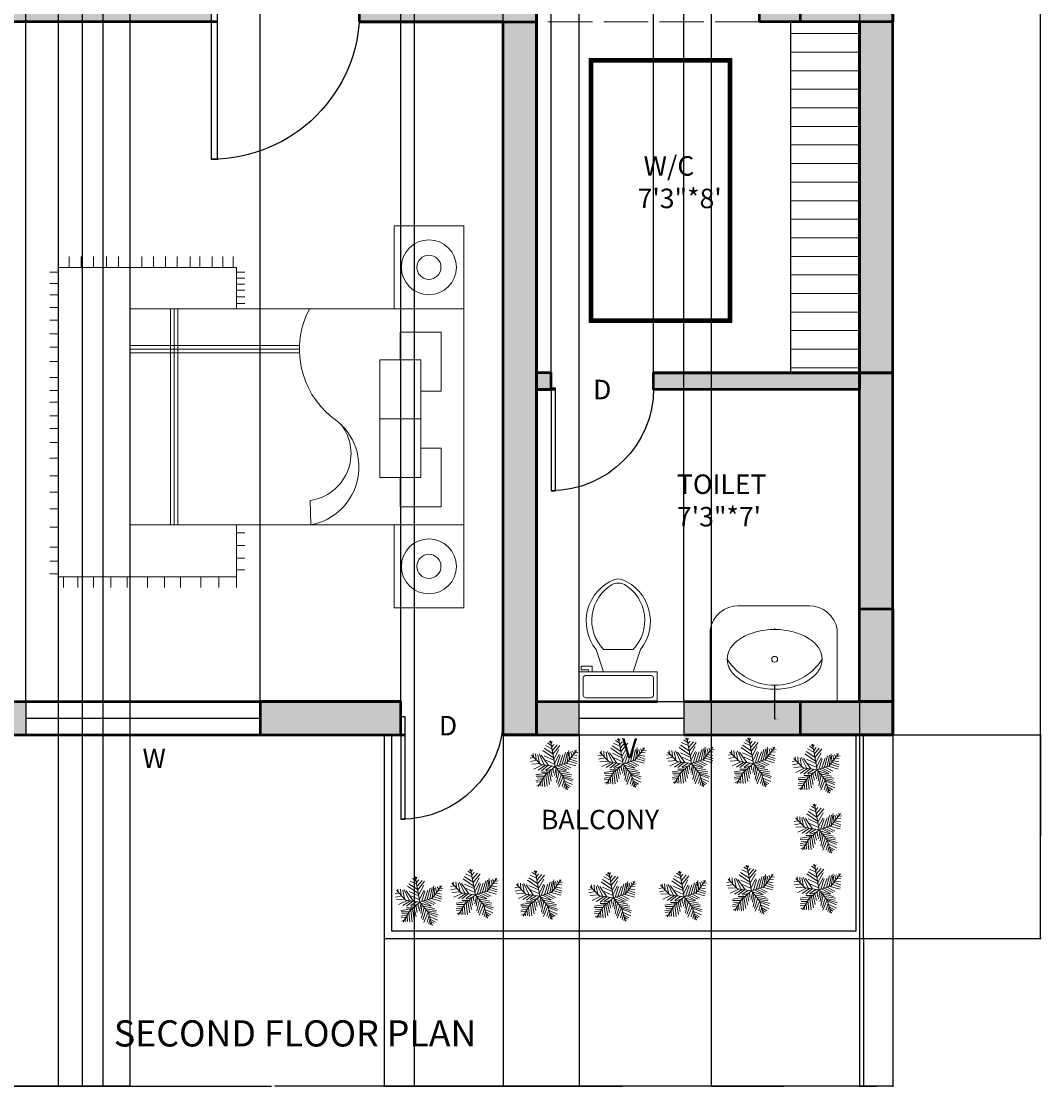
# Model space of a CAD drawing. Units: inches. Extents: x 2494 to 2908, y 1051 to 1885.
# Tile 2 of 7: x 2634 to 2908, y 1051 to 1338. Entities that reach past the tile are written whole.
import ezdxf

# ---------------------------------------------------------------- set-up
doc = ezdxf.new("R2010")
doc.units = ezdxf.units.IN
doc.linetypes.add('ACAD_ISO02W100', pattern=[15, 12, -3])
for name, color, linetype, lineweight in [('A-ANNO-DIMS', 2, 'Continuous', 18), ('A-ANNO-IDEN', 130, 'Continuous', 18), ('A-ANNO-TEXT', 130, 'Continuous', 35), ('A-AREA-IDEN', 130, 'Continuous', 18), ('A-COLS-PATT', 200, 'Continuous', 13), ('A-FLOR-CASE', 230, 'Continuous', 25), ('A-FLOR-FIXT', 230, 'Continuous', 18), ('A-FLOR-HRAL', 140, 'Continuous', 25), ('A-FURN-PATT', 230, 'Continuous', 13), ('A-WALL-OVHD', 140, 'ACAD_ISO02W100', 18), ('A-WALL-PATT', 140, 'Continuous', 13), ('COLUMN', 200, 'Continuous', 50), ('DOOR', 50, 'Continuous', 25), ('FUR', 230, 'Continuous', 18), ('TREE', 100, 'Continuous', 13), ('WALL', 140, 'Continuous', 50), ('WIND', 210, 'Continuous', 25)]:
    doc.layers.add(name, color=color, linetype=linetype, lineweight=lineweight)
doc.styles.get("Standard").update_dxf_attribs({"font": 'arial.ttf'})
doc.dimstyles.get("Standard").update_dxf_attribs({"dimtxt": 0.18, "dimasz": 0.18, "dimexe": 0.18, "dimexo": 0.0625, "dimgap": 0.09, "dimtad": 0, "dimtih": 1, "dimtoh": 1, "dimdec": 4, "dimzin": 0, "dimdsep": 46, "dimtxsty": 'Standard', "dimcen": 0.09, "dimadec": 0, "dimazin": 0, "dimtfac": 1, "dimtdec": 4, "dimtofl": 0, "dimtmove": 0, "dimatfit": 3, "dimfxl": 1, "dimtolj": 1, "dimtzin": 0, "dimarcsym": 0})

# ---------------------------------------------------------------- blocks, each defined once
blk = doc.blocks.new('*U6')
for p, q in [((-8.737, 47.138), (-17.069, 52.711)), ((-10.186, 53.64), (-13.084, 55.962)), ((0, 0), (-10.5, 57)), ((-9.099, 51.782), (-6.563, 55.962)), ((-7.65, 43.423), (-2.578, 49.46)), ((-5.839, 35.992), (4.667, 48.067)), ((-31.5, 4.5), (-52.5, 25.5)), ((-48.585, 21.131), (-49.309, 29.026)), ((-43.513, 28.561), (-42.427, 15.558)), ((-38.442, 26.239), (-34.819, 7.663)), ((-35.544, 28.097), (-24.314, 3.947)), ((-14.533, 2.09), (-30.834, 25.31)), ((-3.665, 19.273), (-27.574, 35.527)), ((-5.114, 28.097), (-24.676, 40.636)), ((-24.314, 23.917), (-2.941, 13.7)), ((-7.288, 39.707), (-21.778, 46.673)), ((-5.114, 27.632), (10.463, 46.673)), ((-2.941, 16.486), (8.652, 37.85)), ((-1.129, 6.734), (9.014, 26.704)), ((3.942, 1.625), (11.187, 24.381)), ((10.101, 3.483), (17.708, 26.239)), ((16.259, 5.805), (23.142, 31.348)), ((22.055, 7.198), (27.489, 32.277)), ((27, 9), (48, 36)), ((27.127, 9.056), (31.112, 35.992)), ((31.836, 30.883), (32.561, 16.486)), ((35.096, 32.741), (37.27, 22.524)), ((38.719, 34.134), (41.979, 28.561)), ((40.53, 25.775), (48.862, 24.846)), ((43.791, 29.954), (51.036, 30.883)), ((44.153, 36.456), (45.239, 32.741)), ((-47.498, 19.737), (-55.83, 18.344)), ((-40.615, 13.7), (-55.105, 10.913)), ((-33.37, 6.269), (-52.207, 5.34)), ((-28.299, 3.483), (-47.86, -5.805)), ((-21.416, 3.018), (-38.079, -8.128)), ((0, 0), (-31.5, 4.5)), ((-15.982, 2.09), (-30.11, -9.521)), ((0, 0), (-22.5, -19.5)), ((-6.563, 1.161), (-21.416, -8.128)), ((-20.691, 13.7), (-1.129, 4.876)), ((0, 0), (27, 9)), ((0, 0), (18, -22.5)), ((6.478, 1.625), (26.04, -8.592)), ((11.187, 3.483), (30.749, -5.805)), ((18.07, 5.805), (35.096, -3.483)), ((24.229, 7.663), (46.688, 1.625)), ((29.662, 12.307), (48.137, 6.269)), ((33.285, 16.486), (48.862, 10.913)), ((36.183, 19.737), (48.137, 17.88)), ((-17.431, -15.094), (-42.789, -18.809)), ((-24.314, -21.596), (-42.427, -22.06)), ((-22.5, -19.5), (-37.5, -45)), ((-15.257, -12.772), (-30.11, -12.772)), ((-20.691, -18.345), (-17.793, -44.352)), ((-6.563, -5.805), (-19.967, -9.985)), ((-17.069, -15.094), (-12.721, -40.172)), ((-13.446, -11.378), (-8.737, -32.741)), ((-9.461, -8.592), (-6.201, -23.453)), ((-4.752, -3.483), (-3.665, -14.629)), ((2.493, -3.019), (-1.491, -20.202)), ((1.769, -2.555), (24.229, -9.521)), ((5.029, -6.27), (2.131, -25.775)), ((9.014, -11.378), (3.58, -35.992)), ((14.085, -16.951), (6.478, -40.172)), ((7.565, -9.056), (32.198, -14.629)), ((18.07, -22.524), (8.289, -45.745)), ((12.274, -15.094), (36.907, -18.809)), ((16.259, -19.738), (36.183, -22.989)), ((18, -22.5), (27, -52.5)), ((18.433, -22.524), (40.53, -29.026)), ((-28.299, -29.026), (-42.789, -31.348)), ((-30.834, -34.135), (-42.427, -35.528)), ((-34.457, -39.708), (-40.978, -42.494)), ((-26.849, -26.24), (-40.253, -25.775)), ((-32.646, -36.921), (-31.921, -44.352)), ((-29.023, -30.884), (-27.936, -43.887)), ((-25.038, -23.918), (-22.865, -45.281)), ((20.244, -30.419), (15.897, -44.816)), ((19.157, -25.311), (38.719, -33.206)), ((22.78, -37.85), (19.519, -48.532)), ((21.331, -32.741), (39.081, -40.636)), ((22.78, -38.314), (34.372, -44.816)), ((24.591, -45.745), (23.142, -50.854)), ((24.591, -43.423), (30.749, -47.603)), ((26.764, -49.925), (28.213, -50.854))]:
    blk.add_line(p, q)
blk = doc.blocks.new('*U2')
for p, q in [((0, 0), (0, -6)), ((40, 0), (40, -6))]:
    blk.add_line(p, q)
blk.add_lwpolyline([(0, 0), (0, 40), (1.75, 40), (1.75, 0)], close=True)
blk.add_arc((0, 0), 40, 0, 90)
blk = doc.blocks.new('*U4')
for p, q in [((9.5, -6), (9.5, -2)), ((-10, -8.5), (-8, -8.5)), ((-10, -9.5), (-10, -8.5)), ((-8, -8.5), (-8, -8)), ((-7, -8), (-7, -9.5)), ((-4, -8), (-6, -14)), ((4, -8), (6, -14)), ((-7, -9.5), (-10, -9.5)), ((4, -14), (-4, -14))]:
    blk.add_line(p, q)
blk.add_lwpolyline([(10.5, -8), (10.5, 0), (-10.5, 0), (-10.5, -8)], close=True)
for points in [[(-9.5, -2), (-9.5, -6)], [(8.5, -1), (-8.5, -1)], [(-8.5, -7), (8.5, -7)]]:
    blk.add_lwpolyline(points)
for centre, radius, start, end in [((-8.62, -1.88), 0.884, 81.8699, 188.1301), ((8.62, -1.88), 0.884, 351.8699, 98.1301), ((-8.62, -6.12), 0.884, 171.8699, 278.1301), ((8.62, -6.12), 0.884, 261.8699, 8.1301), ((3.52, -21.58), 12.17, 141.4691, 247.9714), ((4.2, -21.82), 11.33, 136.3677, 238.9468), ((-3.52, -21.58), 12.17, 292.0284, 38.5307), ((-4.2, -21.82), 11.33, 301.053, 43.6321), ((0, -27.88), 4, 245.7318, 294.2682), ((0, -29), 4, 254.8605, 285.1395)]:
    blk.add_arc(centre, radius, start, end)
blk = doc.blocks.new('BED-DOUBLE')
for p, q in [((10.93, 58.24), (10.93, 0)), ((11.93, 58.24), (11.93, 0)), ((12.93, 58.24), (12.93, 0)), ((45.66, 48.34), (0, 48.34)), ((45.66, 47.34), (0, 47.34)), ((45.66, 46.34), (0, 46.34)), ((67.33, 28.6), (78.31, 28.6)), ((48.68, 0), (48.5, 6.63))]:
    blk.add_line(p, q)
for points in [[(89.88, 0), (0, 0), (0, 58.24), (89.88, 58.24)], [(78.31, 44.44), (67.33, 44.44), (67.33, 12.76), (78.31, 12.76)], [(67.33, 28.6), (78.31, 28.6), (78.31, 44.44), (67.33, 44.44)], [(67.33, 12.76), (78.31, 12.76), (78.31, 28.6), (67.33, 28.6)]]:
    blk.add_lwpolyline(points, close=True)
for points in [[(78.31, 36.06), (83.8, 36.06), (83.8, 51.9), (72.82, 51.9), (72.82, 44.44)], [(72.82, 12.76), (72.82, 4.84), (83.8, 4.84), (83.8, 20.68), (78.31, 20.68)]]:
    blk.add_lwpolyline(points)
for centre, radius, start, end in [((69.31, 47.34), 23.65, 152.5545, 230.8062), ((45.78, 15.63), 15.89, 280.497, 57.3115), ((46.81, 19.24), 12.73, 277.6511, 37.2925)]:
    blk.add_arc(centre, radius, start, end)
blk = doc.blocks.new('NIGHTSTAND-WITH-LAMP')
blk.add_lwpolyline([(18.73, 0), (0, 0), (0, 22.3), (18.73, 22.3)], close=True)
for radius in [7.4, 3.25]:
    blk.add_circle((9.36, 11.15), radius)
blk = doc.blocks.new('RUG-BEDROOM-FRINGED')
for p, q in [((5.18, 86.18), (5.18, 89.12)), ((8.36, 86.18), (8.36, 89.12)), ((11.73, 86.18), (11.73, 89.12)), ((15.23, 86.18), (15.23, 89.12)), ((18.48, 86.18), (18.48, 89.12)), ((21.53, 86.18), (21.53, 89.12)), ((24.71, 86.18), (24.71, 89.12)), ((27.86, 86.18), (27.86, 89.12)), ((31.13, 86.18), (31.13, 89.12)), ((34.27, 86.18), (34.27, 89.12)), ((37.78, 86.18), (37.78, 89.12)), ((40.38, 86.18), (40.38, 89.12)), ((43.7, 86.18), (43.7, 89.12)), ((46.57, 86.18), (46.57, 89.12)), ((49.32, 86.18), (49.32, 89.12)), ((50.28, 86.18), (2.23, 86.18)), ((2.23, 86.18), (2.23, 2.94)), ((50.28, 75.11), (50.28, 86.18)), ((0, 84.95), (2.23, 84.95)), ((50.28, 84.95), (52.51, 84.95)), ((50.28, 83.33), (52.51, 83.33)), ((0, 81.88), (2.23, 81.88)), ((50.28, 81.74), (52.51, 81.74)), ((0, 78.8), (2.23, 78.8)), ((50.28, 80.14), (52.51, 80.14)), ((50.28, 78.33), (52.51, 78.33)), ((0, 75.44), (2.23, 75.44)), ((50.28, 76.54), (52.51, 76.54)), ((0, 71.98), (2.23, 71.98)), ((0, 68.3), (2.23, 68.3)), ((0, 64.75), (2.23, 64.75)), ((0, 60.92), (2.23, 60.92)), ((0, 56.55), (2.23, 56.55)), ((0, 53.1), (2.23, 53.1)), ((0, 49.9), (2.23, 49.9)), ((0, 46.27), (2.23, 46.27)), ((0, 42.87), (2.23, 42.87)), ((0, 39.09), (2.23, 39.09)), ((0, 34.84), (2.23, 34.84)), ((0, 30.1), (2.23, 30.1)), ((0, 25.69), (2.23, 25.69)), ((0, 21.25), (2.23, 21.25)), ((0, 16.29), (2.23, 16.29)), ((50.28, 2.94), (50.28, 16.87)), ((50.28, 14.72), (52.51, 14.72)), ((0, 10.85), (2.23, 10.85)), ((50.28, 11.34), (52.51, 11.34)), ((0, 7.08), (2.23, 7.08)), ((50.28, 7.95), (52.51, 7.95)), ((0, 3.73), (2.23, 3.73)), ((2.23, 2.94), (50.28, 2.94)), ((3.63, 0), (3.63, 2.94)), ((7.47, 0), (7.47, 2.94)), ((11.7, 0), (11.7, 2.94)), ((16.39, 0), (16.39, 2.94)), ((20.78, 0), (20.78, 2.94)), ((26.26, 0), (26.26, 2.94)), ((30.86, 0), (30.86, 2.94)), ((35.17, 0), (35.17, 2.94)), ((40.63, 0), (40.63, 2.94)), ((45.48, 0), (45.48, 2.94)), ((50.28, 4.8), (52.51, 4.8)), ((50.28, 0), (50.28, 2.94))]:
    blk.add_line(p, q)
blk = doc.blocks.new('*D25')
at = {"layer": 'A-ANNO-DIMS', "color": 0, "lineweight": -2, "transparency": 16777216}
for p, q in [((2534.4, 1338.09), (2534.4, 1051.41)), ((2868.25, 1146.09), (2868.25, 1051.41)), ((2534.58, 1051.59), (2700.86, 1051.59)), ((2868.07, 1051.59), (2701.79, 1051.59))]:
    blk.add_line(p, q, dxfattribs=at)
at = {"layer": 'A-ANNO-DIMS', "color": 0, "lineweight": 100, "transparency": 16777216}
for points in [[(2534.58, 1051.62), (2534.58, 1051.56), (2534.4, 1051.59)], [(2868.07, 1051.62), (2868.07, 1051.56), (2868.25, 1051.59)]]:
    blk.add_solid(points, dxfattribs=at)
at = {"layer": 'Defpoints', "color": 0, "lineweight": 100, "transparency": 16777216}
for p in [(2534.4, 1338.16), (2868.25, 1146.16), (2868.25, 1051.59)]:
    blk.add_point(p, dxfattribs=at)
at = {"layer": 'A-ANNO-DIMS', "color": 0, "transparency": 16777216, "insert": (2701.33, 1051.59), "char_height": 0.18, "attachment_point": 5}
blk.add_mtext('\\A1;333.85', dxfattribs=at)
blk = doc.blocks.new('*D26')
at = {"layer": 'A-ANNO-DIMS', "color": 0, "lineweight": -2, "transparency": 16777216}
for p, q in [((2868.31, 1845.16), (2908.18, 1845.16)), ((2908, 1844.98), (2908, 1468.43)), ((2908, 1091.52), (2908, 1468.07)), ((2860.37, 1091.34), (2908.18, 1091.34))]:
    blk.add_line(p, q, dxfattribs=at)
at = {"layer": 'A-ANNO-DIMS', "color": 0, "lineweight": 100, "transparency": 16777216}
for points in [[(2907.97, 1844.98), (2908.03, 1844.98), (2908, 1845.16)], [(2907.97, 1091.52), (2908.03, 1091.52), (2908, 1091.34)]]:
    blk.add_solid(points, dxfattribs=at)
at = {"layer": 'Defpoints', "color": 0, "lineweight": 100, "transparency": 16777216}
for p in [(2868.25, 1845.16), (2908, 1845.16), (2860.3, 1091.34)]:
    blk.add_point(p, dxfattribs=at)
at = {"layer": 'A-ANNO-DIMS', "color": 0, "transparency": 16777216, "insert": (2908, 1468.25), "char_height": 0.18, "attachment_point": 5}
blk.add_mtext('\\A1;753.8', dxfattribs=at)
blk = doc.blocks.new('*D30')
at = {"layer": 'A-ANNO-DIMS', "color": 0, "lineweight": -2, "transparency": 16777216}
for p, q in [((2731.2, 1091.28), (2731.2, 1051.41)), ((2860.3, 1091.28), (2860.3, 1051.41)), ((2731.38, 1051.59), (2795.38, 1051.59)), ((2860.12, 1051.59), (2796.12, 1051.59))]:
    blk.add_line(p, q, dxfattribs=at)
at = {"layer": 'A-ANNO-DIMS', "color": 0, "lineweight": 100, "transparency": 16777216}
for points in [[(2731.38, 1051.62), (2731.38, 1051.56), (2731.2, 1051.59)], [(2860.12, 1051.62), (2860.12, 1051.56), (2860.3, 1051.59)]]:
    blk.add_solid(points, dxfattribs=at)
at = {"layer": 'Defpoints', "color": 0, "lineweight": 100, "transparency": 16777216}
for p in [(2731.2, 1091.34), (2860.3, 1091.34), (2860.3, 1051.59)]:
    blk.add_point(p, dxfattribs=at)
at = {"layer": 'A-ANNO-DIMS', "color": 0, "transparency": 16777216, "insert": (2795.75, 1051.59), "char_height": 0.18, "attachment_point": 5}
blk.add_mtext('\\A1;129.1', dxfattribs=at)
blk = doc.blocks.new('*D31')
at = {"layer": 'A-ANNO-DIMS', "color": 0, "lineweight": -2, "transparency": 16777216}
for p, q in [((2868.31, 1146.16), (2908.18, 1146.16)), ((2908, 1145.98), (2908, 1118.93)), ((2908, 1091.52), (2908, 1118.57)), ((2860.37, 1091.34), (2908.18, 1091.34))]:
    blk.add_line(p, q, dxfattribs=at)
at = {"layer": 'A-ANNO-DIMS', "color": 0, "lineweight": 100, "transparency": 16777216}
for points in [[(2907.97, 1145.98), (2908.03, 1145.98), (2908, 1146.16)], [(2907.97, 1091.52), (2908.03, 1091.52), (2908, 1091.34)]]:
    blk.add_solid(points, dxfattribs=at)
at = {"layer": 'Defpoints', "color": 0, "lineweight": 100, "transparency": 16777216}
for p in [(2868.25, 1146.16), (2908, 1146.16), (2860.3, 1091.34)]:
    blk.add_point(p, dxfattribs=at)
at = {"layer": 'A-ANNO-DIMS', "color": 0, "transparency": 16777216, "insert": (2908, 1118.75), "char_height": 0.18, "attachment_point": 5}
blk.add_mtext('\\A1;54.81', dxfattribs=at)
blk = doc.blocks.new('*D32')
at = {"layer": 'A-ANNO-DIMS', "color": 0, "lineweight": -2, "transparency": 16777216}
for p, q in [((2868.25, 1146.09), (2868.25, 1051.41)), ((2860.3, 1091.28), (2860.3, 1051.41)), ((2860.48, 1051.59), (2863.88, 1051.59)), ((2868.07, 1051.59), (2864.67, 1051.59))]:
    blk.add_line(p, q, dxfattribs=at)
at = {"layer": 'A-ANNO-DIMS', "color": 0, "lineweight": 100, "transparency": 16777216}
for points in [[(2860.48, 1051.62), (2860.48, 1051.56), (2860.3, 1051.59)], [(2868.07, 1051.62), (2868.07, 1051.56), (2868.25, 1051.59)]]:
    blk.add_solid(points, dxfattribs=at)
at = {"layer": 'Defpoints', "color": 0, "lineweight": 100, "transparency": 16777216}
for p in [(2868.25, 1146.16), (2860.3, 1091.34), (2868.25, 1051.59)]:
    blk.add_point(p, dxfattribs=at)
at = {"layer": 'A-ANNO-DIMS', "color": 0, "transparency": 16777216, "insert": (2864.28, 1051.59), "char_height": 0.18, "attachment_point": 5}
blk.add_mtext('\\A1;7.948', dxfattribs=at)
blk = doc.blocks.new('*D33')
at = {"layer": 'A-ANNO-DIMS', "color": 0, "lineweight": -2, "transparency": 16777216}
for p, q in [((2697.84, 1155.22), (2697.84, 1885.09)), ((2698.02, 1884.91), (2716.38, 1884.91)), ((2735.54, 1884.91), (2717.17, 1884.91)), ((2735.72, 1155.22), (2735.72, 1885.09))]:
    blk.add_line(p, q, dxfattribs=at)
at = {"layer": 'A-ANNO-DIMS', "color": 0, "lineweight": 100, "transparency": 16777216}
for points in [[(2698.02, 1884.94), (2698.02, 1884.88), (2697.84, 1884.91)], [(2735.54, 1884.94), (2735.54, 1884.88), (2735.72, 1884.91)]]:
    blk.add_solid(points, dxfattribs=at)
at = {"layer": 'Defpoints', "color": 0, "lineweight": 100, "transparency": 16777216}
for p in [(2735.72, 1884.91), (2697.84, 1155.16), (2735.72, 1155.16)]:
    blk.add_point(p, dxfattribs=at)
at = {"layer": 'A-ANNO-DIMS', "color": 0, "transparency": 16777216, "insert": (2716.78, 1884.91), "char_height": 0.18, "attachment_point": 5}
blk.add_mtext('\\A1;37.88', dxfattribs=at)
blk = doc.blocks.new('*D34')
at = {"layer": 'A-ANNO-DIMS', "color": 0, "lineweight": -2, "transparency": 16777216}
for p, q in [((2634.69, 1155.22), (2634.69, 1885.09)), ((2634.87, 1884.91), (2665.87, 1884.91)), ((2697.66, 1884.91), (2666.66, 1884.91)), ((2697.84, 1155.22), (2697.84, 1885.09))]:
    blk.add_line(p, q, dxfattribs=at)
at = {"layer": 'A-ANNO-DIMS', "color": 0, "lineweight": 100, "transparency": 16777216}
for points in [[(2634.87, 1884.94), (2634.87, 1884.88), (2634.69, 1884.91)], [(2697.66, 1884.94), (2697.66, 1884.88), (2697.84, 1884.91)]]:
    blk.add_solid(points, dxfattribs=at)
at = {"layer": 'Defpoints', "color": 0, "lineweight": 100, "transparency": 16777216}
for p in [(2697.84, 1884.91), (2634.69, 1155.16), (2697.84, 1155.16)]:
    blk.add_point(p, dxfattribs=at)
at = {"layer": 'A-ANNO-DIMS', "color": 0, "transparency": 16777216, "insert": (2666.26, 1884.91), "char_height": 0.18, "attachment_point": 5}
blk.add_mtext('\\A1;63.15', dxfattribs=at)
blk = doc.blocks.new('*D35')
at = {"layer": 'A-ANNO-DIMS', "color": 0, "lineweight": -2, "transparency": 16777216}
for p, q in [((2735.72, 1155.22), (2735.72, 1885.09)), ((2735.9, 1884.91), (2749.09, 1884.91)), ((2763.07, 1884.91), (2749.88, 1884.91)), ((2763.25, 1155.22), (2763.25, 1885.09))]:
    blk.add_line(p, q, dxfattribs=at)
at = {"layer": 'A-ANNO-DIMS', "color": 0, "lineweight": 100, "transparency": 16777216}
for points in [[(2735.9, 1884.94), (2735.9, 1884.88), (2735.72, 1884.91)], [(2763.07, 1884.94), (2763.07, 1884.88), (2763.25, 1884.91)]]:
    blk.add_solid(points, dxfattribs=at)
at = {"layer": 'Defpoints', "color": 0, "lineweight": 100, "transparency": 16777216}
for p in [(2763.25, 1884.91), (2735.72, 1155.16), (2763.25, 1155.16)]:
    blk.add_point(p, dxfattribs=at)
at = {"layer": 'A-ANNO-DIMS', "color": 0, "transparency": 16777216, "insert": (2749.49, 1884.91), "char_height": 0.18, "attachment_point": 5}
blk.add_mtext('\\A1;27.53', dxfattribs=at)
blk = doc.blocks.new('*D36')
at = {"layer": 'A-ANNO-DIMS', "color": 0, "lineweight": -2, "transparency": 16777216}
for p, q in [((2763.25, 1146.09), (2763.25, 1051.41)), ((2783.78, 1146.09), (2783.78, 1051.41)), ((2763.43, 1051.59), (2773.12, 1051.59)), ((2783.6, 1051.59), (2773.91, 1051.59))]:
    blk.add_line(p, q, dxfattribs=at)
at = {"layer": 'A-ANNO-DIMS', "color": 0, "lineweight": 100, "transparency": 16777216}
for points in [[(2763.43, 1051.62), (2763.43, 1051.56), (2763.25, 1051.59)], [(2783.6, 1051.62), (2783.6, 1051.56), (2783.78, 1051.59)]]:
    blk.add_solid(points, dxfattribs=at)
at = {"layer": 'Defpoints', "color": 0, "lineweight": 100, "transparency": 16777216}
for p in [(2763.25, 1146.16), (2783.78, 1146.16), (2783.78, 1051.59)]:
    blk.add_point(p, dxfattribs=at)
at = {"layer": 'A-ANNO-DIMS', "color": 0, "transparency": 16777216, "insert": (2773.52, 1051.59), "char_height": 0.18, "attachment_point": 5}
blk.add_mtext('\\A1;20.53', dxfattribs=at)
blk = doc.blocks.new('*D37')
at = {"layer": 'A-ANNO-DIMS', "color": 0, "lineweight": -2, "transparency": 16777216}
for p, q in [((2783.78, 1155.22), (2783.78, 1885.09)), ((2783.96, 1884.91), (2797.38, 1884.91)), ((2811.73, 1884.91), (2798.31, 1884.91)), ((2811.91, 1155.22), (2811.91, 1885.09))]:
    blk.add_line(p, q, dxfattribs=at)
at = {"layer": 'A-ANNO-DIMS', "color": 0, "lineweight": 100, "transparency": 16777216}
for points in [[(2783.96, 1884.94), (2783.96, 1884.88), (2783.78, 1884.91)], [(2811.73, 1884.94), (2811.73, 1884.88), (2811.91, 1884.91)]]:
    blk.add_solid(points, dxfattribs=at)
at = {"layer": 'Defpoints', "color": 0, "lineweight": 100, "transparency": 16777216}
for p in [(2811.91, 1884.91), (2783.78, 1155.16), (2811.91, 1155.16)]:
    blk.add_point(p, dxfattribs=at)
at = {"layer": 'A-ANNO-DIMS', "color": 0, "transparency": 16777216, "insert": (2797.85, 1884.91), "char_height": 0.18, "attachment_point": 5}
blk.add_mtext('\\A1;28.126', dxfattribs=at)
blk = doc.blocks.new('*D40')
at = {"layer": 'A-ANNO-DIMS', "color": 0, "lineweight": -2, "transparency": 16777216}
for p, q in [((2615.49, 1606.59), (2615.49, 1051.41)), ((2655.49, 1606.59), (2655.49, 1051.41)), ((2615.67, 1051.59), (2635.27, 1051.59)), ((2655.31, 1051.59), (2635.71, 1051.59))]:
    blk.add_line(p, q, dxfattribs=at)
at = {"layer": 'A-ANNO-DIMS', "color": 0, "lineweight": 100, "transparency": 16777216}
for points in [[(2615.67, 1051.62), (2615.67, 1051.56), (2615.49, 1051.59)], [(2655.31, 1051.62), (2655.31, 1051.56), (2655.49, 1051.59)]]:
    blk.add_solid(points, dxfattribs=at)
at = {"layer": 'Defpoints', "color": 0, "lineweight": 100, "transparency": 16777216}
for p in [(2615.49, 1606.66), (2655.49, 1606.66), (2655.49, 1051.59)]:
    blk.add_point(p, dxfattribs=at)
at = {"layer": 'A-ANNO-DIMS', "color": 0, "transparency": 16777216, "insert": (2635.49, 1051.59), "char_height": 0.18, "attachment_point": 5}
blk.add_mtext('\\A1;40', dxfattribs=at)
blk = doc.blocks.new('*D43')
at = {"layer": 'A-ANNO-DIMS', "color": 0, "lineweight": -2, "transparency": 16777216}
for p, q in [((2776.2, 1243.72), (2776.2, 1885.09)), ((2776.38, 1884.91), (2789.53, 1884.91)), ((2803.62, 1884.91), (2790.46, 1884.91)), ((2803.8, 1243.72), (2803.8, 1885.09))]:
    blk.add_line(p, q, dxfattribs=at)
at = {"layer": 'A-ANNO-DIMS', "color": 0, "lineweight": 100, "transparency": 16777216}
for points in [[(2776.38, 1884.94), (2776.38, 1884.88), (2776.2, 1884.91)], [(2803.62, 1884.94), (2803.62, 1884.88), (2803.8, 1884.91)]]:
    blk.add_solid(points, dxfattribs=at)
at = {"layer": 'Defpoints', "color": 0, "lineweight": 100, "transparency": 16777216}
for p in [(2803.8, 1884.91), (2776.2, 1243.66), (2803.8, 1243.66)]:
    blk.add_point(p, dxfattribs=at)
at = {"layer": 'A-ANNO-DIMS', "color": 0, "transparency": 16777216, "insert": (2790, 1884.91), "char_height": 0.18, "attachment_point": 5}
blk.add_mtext('\\A1;27.604', dxfattribs=at)
blk = doc.blocks.new('*D49')
at = {"layer": 'A-ANNO-DIMS', "color": 0, "lineweight": -2, "transparency": 16777216}
for p, q in [((2587.26, 1358.2), (2587.26, 1051.41)), ((2649.88, 1357.95), (2649.88, 1051.41)), ((2587.44, 1051.59), (2618.17, 1051.59)), ((2649.7, 1051.59), (2618.96, 1051.59))]:
    blk.add_line(p, q, dxfattribs=at)
at = {"layer": 'A-ANNO-DIMS', "color": 0, "lineweight": 100, "transparency": 16777216}
for points in [[(2587.44, 1051.62), (2587.44, 1051.56), (2587.26, 1051.59)], [(2649.7, 1051.62), (2649.7, 1051.56), (2649.88, 1051.59)]]:
    blk.add_solid(points, dxfattribs=at)
at = {"layer": 'Defpoints', "color": 0, "lineweight": 100, "transparency": 16777216}
for p in [(2587.26, 1358.26), (2649.88, 1358.01), (2649.88, 1051.59)]:
    blk.add_point(p, dxfattribs=at)
at = {"layer": 'A-ANNO-DIMS', "color": 0, "transparency": 16777216, "insert": (2618.57, 1051.59), "char_height": 0.18, "attachment_point": 5}
blk.add_mtext('\\A1;62.62', dxfattribs=at)
blk = doc.blocks.new('*D53')
at = {"layer": 'A-ANNO-DIMS', "color": 0, "lineweight": -2, "transparency": 16777216}
for p, q in [((2739.28, 1497.29), (2739.28, 1051.41)), ((2819.28, 1497.29), (2819.28, 1051.41)), ((2739.46, 1051.59), (2779.06, 1051.59)), ((2819.1, 1051.59), (2779.5, 1051.59))]:
    blk.add_line(p, q, dxfattribs=at)
at = {"layer": 'A-ANNO-DIMS', "color": 0, "lineweight": 100, "transparency": 16777216}
for points in [[(2739.46, 1051.62), (2739.46, 1051.56), (2739.28, 1051.59)], [(2819.1, 1051.62), (2819.1, 1051.56), (2819.28, 1051.59)]]:
    blk.add_solid(points, dxfattribs=at)
at = {"layer": 'Defpoints', "color": 0, "lineweight": 100, "transparency": 16777216}
for p in [(2739.28, 1497.36), (2819.28, 1497.36), (2819.28, 1051.59)]:
    blk.add_point(p, dxfattribs=at)
at = {"layer": 'A-ANNO-DIMS', "color": 0, "transparency": 16777216, "insert": (2779.28, 1051.59), "char_height": 0.18, "attachment_point": 5}
blk.add_mtext('\\A1;80', dxfattribs=at)
blk = doc.blocks.new('*D56')
at = {"layer": 'A-ANNO-DIMS', "color": 0, "lineweight": -2, "transparency": 16777216}
for p, q in [((2819.28, 1530.09), (2819.28, 1051.41)), ((2859.25, 1530.09), (2859.25, 1051.41)), ((2819.46, 1051.59), (2838.8, 1051.59)), ((2859.07, 1051.59), (2839.73, 1051.59))]:
    blk.add_line(p, q, dxfattribs=at)
at = {"layer": 'A-ANNO-DIMS', "color": 0, "lineweight": 100, "transparency": 16777216}
for points in [[(2819.46, 1051.62), (2819.46, 1051.56), (2819.28, 1051.59)], [(2859.07, 1051.62), (2859.07, 1051.56), (2859.25, 1051.59)]]:
    blk.add_solid(points, dxfattribs=at)
at = {"layer": 'Defpoints', "color": 0, "lineweight": 100, "transparency": 16777216}
for p in [(2819.28, 1530.16), (2859.25, 1530.16), (2859.25, 1051.59)]:
    blk.add_point(p, dxfattribs=at)
at = {"layer": 'A-ANNO-DIMS', "color": 0, "transparency": 16777216, "insert": (2839.26, 1051.59), "char_height": 0.18, "attachment_point": 5}
blk.add_mtext('\\A1;39.975', dxfattribs=at)
blk = doc.blocks.new('*D59')
at = {"layer": 'A-ANNO-DIMS', "color": 0, "lineweight": -2, "transparency": 16777216}
for p, q in [((2859.25, 1530.09), (2859.25, 1051.41)), ((2868.25, 1529.48), (2868.25, 1051.41)), ((2859.43, 1051.59), (2863.6, 1051.59)), ((2868.07, 1051.59), (2863.9, 1051.59))]:
    blk.add_line(p, q, dxfattribs=at)
at = {"layer": 'A-ANNO-DIMS', "color": 0, "lineweight": 100, "transparency": 16777216}
for points in [[(2859.43, 1051.62), (2859.43, 1051.56), (2859.25, 1051.59)], [(2868.07, 1051.62), (2868.07, 1051.56), (2868.25, 1051.59)]]:
    blk.add_solid(points, dxfattribs=at)
at = {"layer": 'Defpoints', "color": 0, "lineweight": 100, "transparency": 16777216}
for p in [(2859.25, 1530.16), (2868.25, 1529.54), (2868.25, 1051.59)]:
    blk.add_point(p, dxfattribs=at)
at = {"layer": 'A-ANNO-DIMS', "color": 0, "transparency": 16777216, "insert": (2863.75, 1051.59), "char_height": 0.18, "attachment_point": 5}
blk.add_mtext('\\A1;9', dxfattribs=at)
blk = doc.blocks.new('*D65')
at = {"layer": 'A-ANNO-DIMS', "color": 0, "lineweight": -2, "transparency": 16777216}
for p, q in [((2662.76, 1694.66), (2662.76, 1051.41)), ((2643.46, 1680.73), (2643.46, 1051.41)), ((2643.64, 1051.59), (2652.66, 1051.59)), ((2662.58, 1051.59), (2653.57, 1051.59))]:
    blk.add_line(p, q, dxfattribs=at)
at = {"layer": 'A-ANNO-DIMS', "color": 0, "lineweight": 100, "transparency": 16777216}
for points in [[(2643.64, 1051.62), (2643.64, 1051.56), (2643.46, 1051.59)], [(2662.58, 1051.62), (2662.58, 1051.56), (2662.76, 1051.59)]]:
    blk.add_solid(points, dxfattribs=at)
at = {"layer": 'Defpoints', "color": 0, "lineweight": 100, "transparency": 16777216}
for p in [(2662.76, 1694.72), (2643.46, 1680.79), (2662.76, 1051.59)]:
    blk.add_point(p, dxfattribs=at)
at = {"layer": 'A-ANNO-DIMS', "color": 0, "transparency": 16777216, "insert": (2653.11, 1051.59), "char_height": 0.18, "attachment_point": 5}
blk.add_mtext('\\A1;19.305', dxfattribs=at)
blk = doc.blocks.new('*D69')
at = {"layer": 'A-ANNO-DIMS', "color": 0, "lineweight": -2, "transparency": 16777216}
for p, q in [((2836.31, 1174.75), (2836.49, 1174.75)), ((2836.4, 1174.66), (2836.4, 1174.84)), ((2836.4, 1150.41), (2836.4, 1159.36)), ((2836.58, 1150.41), (2836.4, 1150.41))]:
    blk.add_line(p, q, dxfattribs=at)
at = {"layer": 'A-ANNO-DIMS', "color": 0, "lineweight": 100, "transparency": 16777216}
blk.add_solid([(2836.43, 1159.36), (2836.37, 1159.36), (2836.4, 1159.54)], dxfattribs=at)
at = {"layer": 'Defpoints', "color": 0, "lineweight": 100, "transparency": 16777216}
for p in [(2836.4, 1174.75), (2836.4, 1159.54)]:
    blk.add_point(p, dxfattribs=at)
at = {"layer": 'A-ANNO-DIMS', "color": 0, "transparency": 16777216, "insert": (2837.32, 1150.41), "char_height": 0.18, "attachment_point": 5}
blk.add_mtext('\\A1;2X R15.215', dxfattribs=at)

msp = doc.modelspace()

# ---------------------------------------------------------------- hatches: boundary and pattern name
at = {"layer": 'A-COLS-PATT'}
h = msp.add_hatch(color=256, dxfattribs=at)
h.dxf.hatch_style = 1
h.paths.add_polyline_path([(2584.1612, 1845.1561), (2559.2517, 1845.1561), (2559.2517, 1836.1561), (2584.1612, 1836.1561)])
h.paths.add_polyline_path([(2720.7462, 1845.1561), (2695.8368, 1845.1561), (2695.8368, 1836.1561), (2720.7462, 1836.1561)])
h.paths.add_polyline_path([(2868.2517, 1845.1561), (2843.3423, 1845.1561), (2843.3423, 1836.1561), (2868.2517, 1836.1561)])
h.paths.add_polyline_path([(2568.2517, 1728.1561), (2559.2517, 1728.1561), (2559.2517, 1703.2467), (2568.2517, 1703.2467)])
h.paths.add_polyline_path([(2568.2517, 1564.0885), (2559.2517, 1564.0885), (2559.2517, 1539.1791), (2568.2517, 1539.1791)])
h.paths.add_polyline_path([(2868.2517, 1554.4528), (2859.2517, 1554.4528), (2859.2517, 1529.5434), (2868.2517, 1529.5434)])
h.paths.add_polyline_path([(2806.0841, 1611.1561), (2781.1746, 1611.1561), (2781.1746, 1602.1561), (2806.0841, 1602.1561)])
h.paths.add_polyline_path([(2868.0971, 1611.1561), (2843.1877, 1611.1561), (2843.1877, 1602.1561), (2868.0971, 1602.1561)])
h.paths.add_polyline_path([(2584.1612, 1347.1561), (2559.2517, 1347.1561), (2559.2517, 1338.1561), (2584.1612, 1338.1561)])
h.paths.add_polyline_path([(2868.2517, 1347.1561), (2843.3423, 1347.1561), (2843.3423, 1338.1561), (2868.2517, 1338.1561)])
h.paths.add_polyline_path([(2568.2517, 1180.0656), (2559.2517, 1180.0656), (2559.2517, 1155.1561), (2568.2517, 1155.1561)])
h.paths.add_polyline_path([(2584.1612, 1155.1561), (2559.2517, 1155.1561), (2559.2517, 1146.1561), (2584.1612, 1146.1561)])
h.paths.add_polyline_path([(2868.2517, 1155.1561), (2843.3423, 1155.1561), (2843.3423, 1146.1561), (2868.2517, 1146.1561)])
h.paths.add_polyline_path([(2868.2517, 1180.0656), (2859.2517, 1180.0656), (2859.2517, 1155.1561), (2868.2517, 1155.1561)])
at = {"layer": 'A-FURN-PATT'}
h = msp.add_hatch(dxfattribs=at)
h.set_pattern_fill('ACAD_ISO04W100', color=256)
h.paths.add_polyline_path([(2763.2517, 1836.1561), (2568.2517, 1836.1561), (2568.2517, 1811.916), (2763.2517, 1811.916)])
h.paths.add_polyline_path([(2859.2517, 1836.1561), (2843.3423, 1836.1561), (2832.2996, 1836.1561), (2832.2996, 1687.6561), (2859.2517, 1687.6561)])
h.paths.add_polyline_path([(2859.2517, 1338.1485), (2840.7638, 1338.1485), (2840.7638, 1243.6561), (2859.2517, 1243.6561)])
at = {"layer": 'A-WALL-PATT'}
h = msp.add_hatch(color=256, dxfattribs=at)
h.dxf.hatch_style = 1
h.paths.add_polyline_path([(2868.2517, 1836.1561), (2859.2517, 1836.1561), (2859.2517, 1611.1561), (2868.2517, 1611.1561)])
h.paths.add_polyline_path([(2715.2517, 1611.1561), (2655.4916, 1611.1561), (2655.4916, 1606.6561), (2715.2517, 1606.6561)])
h.paths.add_polyline_path([(2781.1746, 1611.1561), (2776.9029, 1611.1561), (2715.2517, 1611.1561), (2715.2517, 1606.6561), (2715.2517, 1602.1561), (2781.1746, 1602.1561)])
h.paths.add_polyline_path([(2868.0971, 1602.1561), (2859.2517, 1602.1561), (2859.2517, 1554.4528), (2868.0971, 1554.4528)])
h.paths.add_polyline_path([(2868.2517, 1529.5434), (2859.2517, 1529.5434), (2859.2517, 1347.1561), (2868.2517, 1347.1561)])
h.paths.add_polyline_path([(2868.2517, 1338.1561), (2859.2517, 1338.1561), (2859.2517, 1243.6561), (2868.2517, 1243.6561)])
h.paths.add_polyline_path([(2568.2517, 1338.1561), (2559.2517, 1338.1561), (2559.2517, 1180.0656), (2568.2517, 1180.0656)])
h.paths.add_polyline_path([(2735.7191, 1155.1561), (2697.838, 1155.1561), (2697.838, 1146.1561), (2735.7191, 1146.1561), (2735.7191, 1151.0155)])
h = msp.add_hatch(color=256, dxfattribs=at)
h.dxf.hatch_style = 1
h.paths.add_polyline_path([(2805.2517, 1547.9123), (2796.2517, 1547.9123), (2796.2517, 1530.1561), (2859.2517, 1530.1561), (2859.2517, 1539.1561), (2805.2517, 1539.1561)])
h.paths.add_polyline_path([(2568.2517, 1606.6561), (2615.4916, 1606.6561), (2615.4916, 1611.1561), (2559.2517, 1611.1561), (2559.2517, 1564.0885), (2568.2517, 1564.0885)])
h.paths.add_polyline_path([(2568.2517, 1539.1791), (2559.2517, 1539.1791), (2559.2517, 1456.6561), (2534.4016, 1456.6561), (2534.4016, 1338.1561), (2559.2517, 1338.1561), (2559.2517, 1342.6561), (2543.4016, 1342.6561), (2543.4016, 1452.1561), (2559.2517, 1452.1561), (2568.2517, 1452.1561), (2674.7517, 1452.1561), (2674.7517, 1456.6561), (2568.2517, 1456.6561)])
h.paths.add_polyline_path([(2684.6403, 1347.1561), (2674.7517, 1347.1561), (2584.1612, 1347.1561), (2584.1612, 1338.1561), (2684.6403, 1338.1561), (2684.6403, 1341.1561)])
h.paths.add_polyline_path([(2843.3423, 1347.1561), (2832.3482, 1347.1561), (2832.3482, 1338.1485), (2843.3423, 1338.1485)])
h.paths.add_polyline_path([(2634.6908, 1155.1561), (2584.1612, 1155.1561), (2584.1612, 1146.1561), (2634.6908, 1146.1561)])
h.paths.add_polyline_path([(2783.7833, 1155.1561), (2772.2517, 1155.1561), (2772.2517, 1146.1561), (2783.7833, 1146.1561)])
h.paths.add_polyline_path([(2843.3423, 1155.1561), (2819.0012, 1155.1561), (2811.9091, 1155.1561), (2811.9091, 1146.1561), (2843.3423, 1146.1561)])
h.paths.add_polyline_path([(2868.2517, 1243.6561), (2859.2517, 1243.6561), (2859.2517, 1239.1561), (2859.2517, 1180.0656), (2868.2517, 1180.0656)])
h = msp.add_hatch(color=256, dxfattribs=at)
h.dxf.hatch_style = 1
h.paths.add_polyline_path([(2772.2517, 1338.1561), (2763.2517, 1338.1561), (2763.2517, 1146.1561), (2772.2517, 1146.1561)])
h.paths.add_polyline_path([(2772.2517, 1347.1561), (2724.6403, 1347.1561), (2724.6403, 1341.1561, -0.01876983), (2724.5277, 1338.1561), (2772.2517, 1338.1561)])
h.paths.add_polyline_path([(2808.4276, 1199.3021), (2836.8916, 1199.3021), (2836.8916, 1218.8855), (2808.4276, 1218.8855)], flags=9)
h.paths.add_polyline_path([(2797.835, 1285.0138), (2820.947, 1285.0138), (2820.947, 1304.5973), (2797.835, 1304.5973)], flags=9)
h = msp.add_hatch(color=256, dxfattribs=at)
h.dxf.hatch_style = 1
h.paths.add_polyline_path([(2859.2517, 1243.6561), (2803.8003, 1243.6561), (2803.8003, 1239.5155), (2803.8003, 1239.1561), (2859.2517, 1239.1561)])
h.paths.add_polyline_path([(2776.196, 1243.6561), (2772.2517, 1243.6561), (2772.2517, 1239.1561), (2776.196, 1239.1561), (2776.196, 1239.5155)])

# ---------------------------------------------------------------- linework, layer by layer
at = {"layer": 'A-FLOR-CASE'}
msp.add_line((2840.7638, 1243.6561), (2840.7638, 1338.1485), dxfattribs=at)
at = {"layer": 'A-FLOR-FIXT'}
for points in [[(2826.5093, 1180.9217), (2845.7646, 1180.9217)], [(2853.2727, 1174.4567), (2853.2727, 1155.1561), (2819.0012, 1155.1561), (2819.0012, 1174.4567)]]:
    msp.add_lwpolyline(points, dxfattribs=at)
msp.add_circle((2836.3955, 1166.5091), 0.7921, dxfattribs=at)
for centre, radius, start, end in [((2826.6193, 1173.2017), 7.7207, 89.183797, 170.645503), ((2845.6546, 1173.2017), 7.7207, 9.354497, 90.816203), ((2836.3955, 1174.753), 15.2147, 212.808997, 327.191003)]:
    msp.add_arc(centre, radius, start, end, dxfattribs=at)
msp.add_ellipse((2836.3955, 1166.5091), major_axis=(12.7877, 0), ratio=0.62936955, dxfattribs=at)
at = {"layer": 'A-FLOR-HRAL'}
for p, q in [((2731.1999, 1146.1561), (2731.1999, 1091.3437)), ((2733.1999, 1146.1561), (2733.1999, 1093.3437)), ((2858.3038, 1093.3437), (2858.3038, 1146.1561)), ((2860.3038, 1091.3437), (2860.3038, 1146.1561)), ((2733.1999, 1093.3437), (2858.3038, 1093.3437)), ((2731.1999, 1091.3437), (2860.3038, 1091.3437))]:
    msp.add_line(p, q, dxfattribs=at)
at = {"layer": 'A-WALL-OVHD'}
msp.add_lwpolyline([(2772.2517, 1347.1561), (2832.3482, 1347.1561), (2832.3482, 1338.1485), (2772.2517, 1338.1485)], close=True, dxfattribs=at)
at = {"layer": 'COLUMN'}
for points in [[(2843.3423, 1347.1561), (2868.2517, 1347.1561), (2868.2517, 1338.1561), (2843.3423, 1338.1561)], [(2868.2517, 1180.0656), (2868.2517, 1155.1561), (2859.2517, 1155.1561), (2859.2517, 1180.0656)], [(2843.3423, 1155.1561), (2868.2517, 1155.1561), (2868.2517, 1146.1561), (2843.3423, 1146.1561)]]:
    msp.add_lwpolyline(points, close=True, dxfattribs=at)
at = {"layer": 'FUR'}
for points in [[(2786.4209, 1328.2863), (2824.8875, 1328.2863), (2824.8875, 1257.2237), (2786.4209, 1257.2237)], [(2786.6709, 1328.0363), (2824.6375, 1328.0363), (2824.6375, 1257.4737), (2786.6709, 1257.4737)], [(2786.9209, 1327.7863), (2824.3875, 1327.7863), (2824.3875, 1257.7237), (2786.9209, 1257.7237)], [(2787.1709, 1327.5363), (2824.1375, 1327.5363), (2824.1375, 1257.9737), (2787.1709, 1257.9737)], [(2787.4209, 1327.2863), (2823.8875, 1327.2863), (2823.8875, 1258.2237), (2787.4209, 1258.2237)]]:
    msp.add_lwpolyline(points, close=True, dxfattribs=at)
at = {"layer": 'WALL'}
for p, q in [((2772.2517, 1146.1561), (2772.2517, 1347.1561)), ((2868.2517, 1243.6561), (2868.2517, 1347.1561)), ((2686.3903, 1338.1561), (2568.2517, 1338.1561)), ((2763.2517, 1338.1561), (2724.5277, 1338.1561)), ((2763.2517, 1155.1561), (2763.2517, 1338.1561)), ((2859.2517, 1338.1485), (2832.3482, 1338.1485)), ((2859.2517, 1243.6561), (2859.2517, 1338.1485)), ((2776.196, 1243.6561), (2772.2517, 1243.6561)), ((2868.2517, 1243.6561), (2803.8003, 1243.6561)), ((2859.2517, 1239.1561), (2859.2517, 1243.6561)), ((2868.2517, 1146.1561), (2868.2517, 1243.6561)), ((2777.4037, 1239.1561), (2772.2517, 1239.1561)), ((2859.2517, 1239.1561), (2803.798, 1239.1561)), ((2859.2517, 1155.1561), (2859.2517, 1239.1561)), ((2568.2517, 1155.1561), (2735.7191, 1155.1561)), ((2772.2517, 1155.1561), (2804.7833, 1155.1561)), ((2811.9091, 1155.1561), (2859.2517, 1155.1561)), ((2559.2517, 1146.1561), (2736.9268, 1146.1561)), ((2762.8923, 1146.1561), (2772.2517, 1146.1561)), ((2772.2517, 1146.1561), (2783.7833, 1146.1561)), ((2811.9091, 1146.1561), (2868.2517, 1146.1561))]:
    msp.add_line(p, q, dxfattribs=at)
for points in [[(2724.5277, 1338.1561), (2772.2517, 1338.1561), (2772.2517, 1347.1561), (2724.5277, 1347.1561)], [(2772.2517, 1146.1561), (2763.2517, 1146.1561), (2763.2517, 1338.1561), (2772.2517, 1338.1561)], [(2859.2517, 1243.6561), (2868.2517, 1243.6561), (2868.2517, 1338.1561), (2859.2517, 1338.1561)], [(2772.2517, 1239.1561), (2776.196, 1239.1561), (2776.196, 1243.6561), (2772.2517, 1243.6561)], [(2859.2517, 1239.1561), (2803.8003, 1239.1561), (2803.8003, 1243.6561), (2859.2517, 1243.6561)], [(2697.838, 1146.1561), (2735.7191, 1146.1561), (2735.7191, 1155.1561), (2697.838, 1155.1561)]]:
    msp.add_lwpolyline(points, close=True, dxfattribs=at)
for points in [[(2772.2517, 1347.1561), (2772.2517, 1338.1485)], [(2832.3482, 1338.1485), (2832.3482, 1347.1561)]]:
    msp.add_lwpolyline(points, dxfattribs=at)
at = {"layer": 'WIND'}
for p, q in [((2783.7833, 1155.1561), (2811.9091, 1155.1561)), ((2634.6908, 1150.6561), (2697.838, 1150.6561)), ((2783.7833, 1150.6561), (2811.9091, 1150.6561)), ((2783.7833, 1146.1561), (2811.9091, 1146.1561))]:
    msp.add_line(p, q, dxfattribs=at)
msp.add_lwpolyline([(2634.6908, 1146.1561), (2697.838, 1146.1561), (2697.838, 1155.1561), (2634.6908, 1155.1561)], close=True, dxfattribs=at)
for points in [[(2783.7833, 1146.1561), (2783.7833, 1155.1561), (2804.7833, 1155.1561)], [(2811.9091, 1155.1561), (2811.9091, 1146.1561)]]:
    msp.add_lwpolyline(points, dxfattribs=at)

# ---------------------------------------------------------------- block references
at = {"layer": 'A-FLOR-FIXT', "xscale": -1, "rotation": 180}
msp.add_blockref('*U4', (2794.2833, 1155.1561), dxfattribs=at)
at = {"layer": 'DOOR', "xscale": -1, "rotation": 180}
msp.add_blockref('*U2', (2684.6403, 1341.1561), dxfattribs=at)
at = {"layer": 'DOOR', "xscale": -0.6901078009918955, "yscale": 0.6901078009918955, "zscale": 0.6901078009918955, "rotation": 180}
for p in [(2776.196, 1239.5155), (2735.7191, 1151.0155)]:
    msp.add_blockref('*U2', p, dxfattribs=at)
at = {"layer": 'FUR'}
for name, p in [('NIGHTSTAND-WITH-LAMP', (2733.918, 1260.919)), ('RUG-BEDROOM-FRINGED', (2641.229, 1185.811)), ('BED-DOUBLE', (2662.765, 1202.681)), ('NIGHTSTAND-WITH-LAMP', (2733.918, 1180.3801))]:
    msp.add_blockref(name, p, dxfattribs=at)
at = {"layer": 'TREE', "xscale": 0.1203413878223358, "yscale": 0.1203413878223358, "zscale": 0.1203413878223358}
for p in [(2795.6099, 1138.3079), (2813.9632, 1138.4716), (2830.6778, 1138.4716), (2777.2566, 1137.6529), (2847.8531, 1136.7601), (2848.3757, 1120.6255), (2830.1862, 1104.1931), (2848.3757, 1104.4167), (2740.8776, 1101.1422), (2755.7897, 1103.1069), (2773.1598, 1102.7556), (2792.988, 1102.293), (2811.9968, 1102.5724)]:
    msp.add_blockref('*U6', p, dxfattribs=at)

# ---------------------------------------------------------------- texts
at = {"layer": 'A-ANNO-IDEN', "char_height": 5.2482, "attachment_point": 1}
for s, insert in [('D', (2787.4904, 1241.7633)), ('D', (2745.9659, 1151.2579)), ('V', (2795.2559, 1145.2047)), ('W', (2666.1461, 1142.4663))]:
    msp.add_mtext_dynamic_manual_height_columns(s, width=250.978097, gutter_width=26.2409, heights=[0], dxfattribs=dict(at, insert=insert))
at = {"layer": 'A-ANNO-TEXT', "insert": (2658.443, 1069.292), "char_height": 7.052574, "attachment_point": 1}
msp.add_mtext_dynamic_manual_height_columns('SECOND FLOOR PLAN', width=337.267898, gutter_width=35.2629, heights=[0], dxfattribs=at)
at = {"layer": 'A-AREA-IDEN', "char_height": 5.24818, "attachment_point": 1}
for s, insert in [(' W/C\\P7\'3"*8\'', (2799.4943, 1301.9857)), ('TOILET\\P7\'3"*7\'', (2810.0868, 1216.2776)), ('BALCONY', (2773.4581, 1125.9703))]:
    msp.add_mtext_dynamic_manual_height_columns(s, width=250.978097, gutter_width=26.2409, heights=[0], dxfattribs=dict(at, insert=insert))

# ---------------------------------------------------------------- dimensions: what is measured, and where the dimension line sits
at = {"layer": 'A-ANNO-DIMS'}
for base, p1, p2, override, picture, middle in [((2697.838, 1884.9061), (2634.6908, 1155.1561), (2697.838, 1155.1561), {"dimdec": 2, "dimlfac": 1, "dimrnd": 0, "dimzin": 0, "dimdsep": 46, "dimlunit": 2}, '*D34', (2666.2644, 1884.9061)), ((2735.7191, 1884.9061), (2697.838, 1155.1561), (2735.7191, 1155.1561), {"dimdec": 2, "dimlfac": 1, "dimrnd": 0, "dimzin": 0, "dimdsep": 46, "dimlunit": 2}, '*D33', (2716.7785, 1884.9061)), ((2763.2517, 1884.9061), (2735.7191, 1155.1561), (2763.2517, 1155.1561), {"dimdec": 2, "dimlfac": 1, "dimrnd": 0, "dimzin": 0, "dimdsep": 46, "dimlunit": 2}, '*D35', (2749.4854, 1884.9061)), ((2803.8003, 1884.9061), (2776.196, 1243.6561), (2803.8003, 1243.6561), {"dimdec": 3, "dimlfac": 1, "dimrnd": 0, "dimzin": 0, "dimdsep": 46, "dimlunit": 2}, '*D43', (2789.9982, 1884.9061)), ((2811.9091, 1884.9061), (2783.7833, 1155.1561), (2811.9091, 1155.1561), {"dimdec": 3, "dimlfac": 1, "dimrnd": 0, "dimzin": 0, "dimdsep": 46, "dimlunit": 2}, '*D37', (2797.8462, 1884.9061)), ((2662.7647, 1051.5937), (2643.4597, 1680.7919), (2662.7647, 1694.719), {"dimdec": 3, "dimlfac": 1, "dimrnd": 0, "dimzin": 0, "dimdsep": 46, "dimlunit": 2}, '*D65', (2653.1122, 1051.5937)), ((2655.4916, 1051.5937), (2615.4916, 1606.6561), (2655.4916, 1606.6561), {"dimdec": 0, "dimlfac": 1, "dimrnd": 0, "dimzin": 0, "dimdsep": 46, "dimlunit": 2}, '*D40', (2635.4916, 1051.5937)), ((2859.2517, 1051.5937), (2819.2763, 1530.1561), (2859.2517, 1530.1561), {"dimdec": 3, "dimlfac": 1, "dimrnd": 0, "dimzin": 0, "dimdsep": 46, "dimlunit": 2}, '*D56', (2839.264, 1051.5937)), ((2868.2517, 1051.5937), (2859.2517, 1530.1561), (2868.2517, 1529.5434), {"dimdec": 0, "dimlfac": 1, "dimrnd": 0, "dimzin": 0, "dimdsep": 46, "dimlunit": 2}, '*D59', (2863.7517, 1051.5937)), ((2819.2763, 1051.5937), (2739.2763, 1497.3573), (2819.2763, 1497.3573), {"dimdec": 0, "dimlfac": 1, "dimrnd": 0, "dimzin": 0, "dimdsep": 46, "dimlunit": 2}, '*D53', (2779.2763, 1051.5937)), ((2649.877, 1051.5937), (2587.2592, 1358.2585), (2649.877, 1358.0085), {"dimdec": 2, "dimlfac": 1, "dimrnd": 0, "dimzin": 0, "dimdsep": 46, "dimlunit": 2}, '*D49', (2618.5681, 1051.5937)), ((2868.2517, 1051.5937), (2534.4016, 1338.1561), (2868.2517, 1146.1561), {"dimdec": 2, "dimlfac": 1, "dimrnd": 0, "dimzin": 0, "dimdsep": 46, "dimlunit": 2}, '*D25', (2701.3267, 1051.5937)), ((2783.7833, 1051.5937), (2763.2517, 1146.1561), (2783.7833, 1146.1561), {"dimdec": 2, "dimlfac": 1, "dimrnd": 0, "dimzin": 0, "dimdsep": 46, "dimlunit": 2}, '*D36', (2773.5175, 1051.5937)), ((2868.2517, 1051.5937), (2860.3038, 1091.3437), (2868.2517, 1146.1561), {"dimdec": 3, "dimlfac": 1, "dimrnd": 0, "dimzin": 0, "dimdsep": 46, "dimlunit": 2}, '*D32', (2864.2778, 1051.5937)), ((2860.3038, 1051.5937), (2731.1999, 1091.3437), (2860.3038, 1091.3437), {"dimdec": 1, "dimlfac": 1, "dimrnd": 0, "dimzin": 0, "dimdsep": 46, "dimlunit": 2}, '*D30', (2795.7519, 1051.5937))]:
    dim = msp.add_linear_dim(base=base, p1=p1, p2=p2, dimstyle='Standard', override=override, dxfattribs=at)
    dim.commit()
    dim.dimension.update_dxf_attribs({"geometry": picture, "text_midpoint": middle})
for base, p2, override, picture, middle in [((2908.0017, 1845.1561), (2868.2517, 1845.1561), {"dimdec": 1, "dimlfac": 1, "dimrnd": 0, "dimzin": 0, "dimdsep": 46, "dimlunit": 2}, '*D26', (2908.0017, 1468.2499)), ((2908.0017, 1146.1561), (2868.2517, 1146.1561), {"dimdec": 2, "dimlfac": 1, "dimrnd": 0, "dimzin": 0, "dimdsep": 46, "dimlunit": 2}, '*D31', (2908.0017, 1118.7499))]:
    dim = msp.add_linear_dim(base=base, p1=(2860.3038, 1091.3437), p2=p2, angle=90, dimstyle='Standard', override=override, dxfattribs=at)
    dim.commit()
    dim.dimension.update_dxf_attribs({"geometry": picture, "text_midpoint": middle})
dim = msp.add_radius_dim(center=(2836.3955, 1174.753), mpoint=(2836.396, 1159.5383), text='2X <>', dimstyle='Standard', override={"dimdec": 3, "dimlfac": 1, "dimrnd": 0, "dimzin": 0, "dimdsep": 46, "dimlunit": 2}, dxfattribs=at)
dim.commit()
dim.dimension.update_dxf_attribs({"geometry": '*D69', "text_midpoint": (2837.3216, 1150.4095), "dimtype": 164})

doc.saveas('drawing.dxf')
